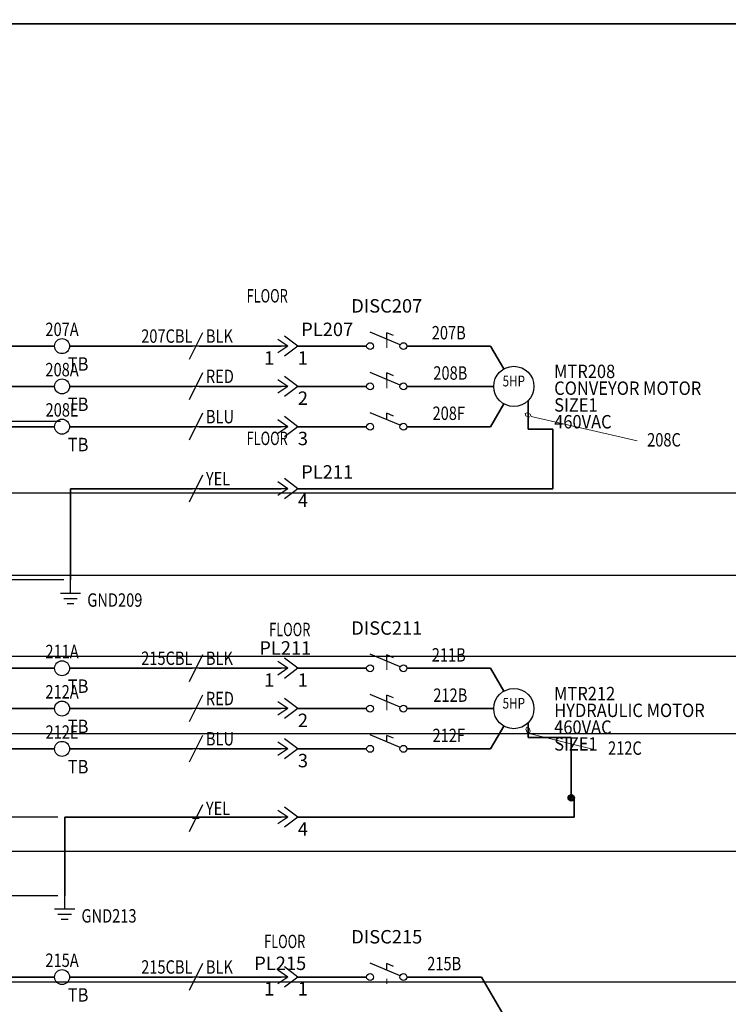
# Model space of a CAD drawing. Extents: x 0 to 33.5, y 0 to 22.4.
# Tile 4 of 8: x 13.3 to 19.9, y 8.5 to 17.7. Entities that reach past the tile are written whole.
import ezdxf
from ezdxf.enums import TextEntityAlignment as Align

# ---------------------------------------------------------------- set-up
doc = ezdxf.new("R2010")
doc.units = 0
doc.header["$MEASUREMENT"] = 0
for name, color, linetype, lineweight in [('A-ANNO-DIMS', 2, 'Continuous', 18), ('LINK', 9, 'Continuous', 18), ('MISC', 7, 'Continuous', 13), ('SYMS', 7, 'Continuous', 25), ('WIRENO', 72, 'Continuous', 18), ('WIRES', 7, 'Continuous', 35)]:
    doc.layers.add(name, color=color, linetype=linetype, lineweight=lineweight)
for name, color, linetype in [('DESC', 150, 'Continuous'), ('DESCCHILD', 20, 'Continuous'), ('TAGS', 150, 'Continuous'), ('TERMS', 123, 'Continuous'), ('WIREREF', 52, 'Continuous')]:
    doc.layers.add(name, color=color, linetype=linetype)
doc.styles.add('WD', font='romans.shx')
doc.dimstyles.get("Standard").update_dxf_attribs({"dimtxt": 0.18, "dimasz": 0.18, "dimexe": 0.18, "dimexo": 0.0625, "dimgap": 0.09, "dimtad": 0, "dimtih": 1, "dimtoh": 1, "dimdec": 4, "dimzin": 0, "dimdsep": 46, "dimtxsty": 'Standard', "dimcen": 0.09, "dimadec": 0, "dimazin": 0, "dimtfac": 1, "dimtdec": 4, "dimtofl": 0, "dimtmove": 0, "dimatfit": 3, "dimfxl": 1, "dimtolj": 1, "dimtzin": 0, "dimarcsym": 0})

# ---------------------------------------------------------------- blocks, each defined once
blk = doc.blocks.new('HT0W02')
blk.add_circle((0, 0), 0.0699)
at = {"style": 'WD'}
for tag, p, width in [('INST', (0.0625, 0.4196), 0.7), ('LOC', (0.0625, 0.25), 0.7), ('DESC1', (0.0532, -0.3851), 0.8)]:
    blk.add_attdef(tag, p, '', height=0.125, dxfattribs=dict(at, width=width))
at = {"style": 'WD', "width": 0.8, "flags": 8}
blk.add_attdef('WIRENO', text='', height=0.125, dxfattribs=at).set_placement((0, 0.0938), align=Align.CENTER)
at = {"style": 'WD', "flags": 1}
for tag, p, height in [('X4TERM01', (-0.0699, 0), 0.0125), ('X4TERMDESC01', (-0.0552, -0.0229), 0.025), ('X2TERMDESC01', (-0.006, 0.0287), 0.025), ('STRIPSEQ', (0, 0), 0.00125), ('X2TERM01', (0, 0.0699), 0.0125), ('X1TERMDESC01', (0.0393, -0.0027), 0.025), ('X1TERM01', (0.0699, 0), 0.0125), ('LINKTERM', (0, -0.0019), 0.00125), ('X8TERM01', (0, -0.0699), 0.0125), ('X8TERMDESC01', (0, -0.0535), 0.025)]:
    blk.add_attdef(tag, p, '', height=height, dxfattribs=at)
at = {"style": 'WD'}
for tag, p, height, width, flags in [('TAGSTRIP', (0.0532, -0.2288), 0.125, 0.9, 8), ('ASSYCODE', (0.0625, -0.2812), 0.01, 0.7, 1), ('CAT', (0.2132, -0.4063), 0.1094, 0.8, 1), ('DESC2', (0.0532, -0.5413), 0.125, 0.8, 8), ('DESC3', (0.0532, -0.6976), 0.125, 0.8, 8)]:
    blk.add_attdef(tag, p, '', height=height, dxfattribs=dict(at, width=width, flags=flags))
at = {"style": 'WD', "width": 0.8, "flags": 1}
blk.add_attdef('MFG', text='', height=0.1094, dxfattribs=at).set_placement((0.0882, -0.4063), align=Align.RIGHT)
blk = doc.blocks.new('HMO13')
blk.add_circle((0, 0), 0.1875)
at = {"style": 'WD'}
for tag, p, width in [('INST', (0.3805, 0.4032), 0.7), ('LOC', (0.3805, 0.2336), 0.7), ('TAG1', (0.375, 0.0774), 0.9), ('DESC1', (0.376, -0.0789), 0.9), ('DESC2', (0.376, -0.2351), 0.9), ('DESC3', (0.376, -0.3914), 0.9), ('RATING3', (0.375, -0.5476), 0.8), ('RATING4', (0.375, -0.7039), 0.8), ('WDTAGALT', (0.375, -0.875), 0.7)]:
    blk.add_attdef(tag, p, '', height=0.125, dxfattribs=dict(at, width=width))
at = {"style": 'WD', "width": 0.8}
blk.add_attdef('RATING1', text='', height=0.1, dxfattribs=at).set_placement((0, 0), align=Align.CENTER)
at = {"style": 'WD', "flags": 1}
for tag, p in [('X0TERM01', (-0.0938, 0.1624)), ('X4TERM02', (-0.1875, 0)), ('X0TERM03', (-0.0938, -0.1624)), ('X0TERM04', (0.1326, -0.1326))]:
    blk.add_attdef(tag, p, '', height=0.0125, dxfattribs=at)
at = {"style": 'WD', "flags": 9}
for tag, p in [('ASSYCODE', (0, 0.125)), ('FAMILY', (-0.0053, 0.1698))]:
    blk.add_attdef(tag, text='', height=0.01, dxfattribs=at).set_placement(p, align=Align.CENTER)
at = {"style": 'WD', "flags": 1}
for tag, p in [('MFG', (0, 0.1404)), ('CAT', (0, 0.1593))]:
    blk.add_attdef(tag, text='', height=0.01, dxfattribs=at).set_placement(p, align=Align.MIDDLE)
at = {"style": 'WD', "width": 0.8}
blk.add_attdef('RATING2', text='', height=0.1, dxfattribs=at).set_placement((0, -0.0312), align=Align.TOP_CENTER)
blk = doc.blocks.new('HDS11')
for p, q in [((0.1257, 0.0127), (-0.1559, 0.1301)), ((0, 0.0651), (0, 0.125)), ((0.0625, 0.099), (0, 0.125))]:
    blk.add_line(p, q)
for centre in [(-0.1553, 0), (0.1553, 0)]:
    blk.add_circle(centre, 0.0322)
at = {"style": 'WD', "width": 0.7}
for tag, p in [('INST', (0, 0.625)), ('LOC', (0, 0.4688)), ('RATING1', (0, 0.1562)), ('XREF', (0, -0.2363)), ('DESC1', (0, -0.4062)), ('DESC2', (0, -0.5625))]:
    blk.add_attdef(tag, text='', height=0.125, dxfattribs=at).set_placement(p, align=Align.CENTER)
at = {"style": 'WD'}
blk.add_attdef('TAG1', text='', height=0.125, dxfattribs=at).set_placement((0, 0.3125), align=Align.CENTER)
for tag, p in [('X2LINK', (0, 0.4375)), ('X8LINK', (0, -0.0156))]:
    blk.add_attdef(tag, p, '', height=0.01, dxfattribs=at)
for tag, p, height, flags in [('FAMILY', (0.2062, 0.1306), 0.01, 9), ('X4TERM01', (-0.1875, 0), 0.0125, 1), ('X1TERM02', (0.1875, 0), 0.0125, 1), ('CONTACT', (0.2062, 0.0401), 0.01, 9)]:
    blk.add_attdef(tag, p, '', height=height, dxfattribs=dict(at, flags=flags))
at = {"style": 'WD', "flags": 9}
for tag, p in [('MFG', (0.2278, 0.0887)), ('CAT', (0.2297, 0.1082)), ('ASSYCODE', (0.2188, 0.0625))]:
    blk.add_attdef(tag, text='', height=0.01, dxfattribs=at).set_placement(p, align=Align.CENTER)
at = {"style": 'WD', "flags": 8}
blk.add_attdef('TERM01', text='', height=0.125, dxfattribs=at).set_placement((-0.25, -0.0314), align=Align.TOP_RIGHT)
blk.add_attdef('TERM02', text='', height=0.125, dxfattribs=at).set_placement((0.25, -0.0314), align=Align.TOP_LEFT)
blk = doc.blocks.new('WDDOT')
for radius in [0.03, 0.0187, 0.00929]:
    blk.add_circle((0, 0), radius)
blk = doc.blocks.new('VGND2')
for p, q in [((0, -0.125), (0, 0)), ((0.09375, -0.125), (-0.09375, -0.125)), ((-0.0625, -0.171875), (0.0625, -0.171875)), ((-0.03125, -0.21875), (0.03125, -0.21875))]:
    blk.add_line(p, q)
at = {"style": 'WD', "width": 0.8}
for tag, p in [('INST', (0.15625, 0.125)), ('LOC', (0.15625, -0.03125)), ('TAG1', (0.15625, -0.1875)), ('DESC1', (0.15625, -0.34375)), ('DESC2', (0.15625, -0.5))]:
    blk.add_attdef(tag, text='', height=0.125, dxfattribs=at).set_placement(p, align=Align.MIDDLE_LEFT)
at = {"style": 'WD', "flags": 1}
for tag in ['ASSYCODE', 'X2TERM01', 'CAT', 'MFG', 'FAMILY']:
    blk.add_attdef(tag, (0, 0), '', height=0.01, dxfattribs=at)
blk = doc.blocks.new('HCN1PJ')
for p, q in [((0.0625, 0), (-0.0625, 0.0938)), ((-0.0312, 0), (-0.125, 0.0625)), ((-0.0312, 0), (-0.125, -0.0625)), ((-0.0312, 0), (-0.0938, 0)), ((0.0625, 0), (-0.0625, -0.0938))]:
    blk.add_line(p, q)
at = {"style": 'WD', "width": 0.7}
for tag, p in [('DESC1', (-0.0312, 0.4062)), ('DESC2', (-0.0312, 0.25))]:
    blk.add_attdef(tag, text='', height=0.125, dxfattribs=at).set_placement(p, align=Align.RIGHT)
for tag, p in [('INST', (0.0938, 0.4062)), ('LOC', (0.0938, 0.25))]:
    blk.add_attdef(tag, p, '', height=0.125, dxfattribs=at)
at = {"style": 'WD'}
for tag, p, height in [('TAG1', (0.0938, 0.0938), 0.125), ('X2LINK', (-0.0625, 0.125), 0.01), ('X8LINK', (-0.0625, -0.125), 0.01)]:
    blk.add_attdef(tag, p, '', height=height, dxfattribs=at)
for tag, p, height, flags in [('WDBLKNAM', (0.0484, 0.1036), 0.01, 9), ('FAMILY', (0.0484, 0.1211), 0.01, 9), ('X4TERMDESC01', (-0.1061, 0.0218), 0.01, 1), ('X4TERM01', (-0.0938, 0), 0.0125, 1), ('X1TERM02', (0.0625, 0), 0.0125, 1), ('X1TERMDESC02', (0.0672, 0.0164), 0.01, 1)]:
    blk.add_attdef(tag, p, '', height=height, dxfattribs=dict(at, flags=flags))
at = {"style": 'WD', "flags": 9}
for tag, p in [('ASSYCODE', (0.0668, 0.0437)), ('MFG', (0.0715, 0.0575)), ('CAT', (0.0735, 0.0769))]:
    blk.add_attdef(tag, text='', height=0.01, dxfattribs=at).set_placement(p, align=Align.CENTER)
at = {"style": 'WD', "flags": 8}
blk.add_attdef('TERM01', text='', height=0.125, dxfattribs=at).set_placement((-0.1562, -0.047), align=Align.TOP_RIGHT)
blk.add_attdef('TERM02', text='', height=0.125, dxfattribs=at).set_placement((0.0625, -0.047), align=Align.TOP_LEFT)
blk = doc.blocks.new('HCN2PJ')
for p, q in [((0.0625, 0), (-0.0625, 0.0938)), ((-0.0312, 0), (-0.125, 0.0625)), ((-0.0312, 0), (-0.125, -0.0625)), ((-0.0312, 0), (-0.0938, 0)), ((0.0625, 0), (-0.0625, -0.0938))]:
    blk.add_line(p, q)
at = {"style": 'WD', "width": 0.7}
for tag, p in [('DESC1', (-0.0312, 0.4062)), ('DESC2', (-0.0312, 0.25))]:
    blk.add_attdef(tag, text='', height=0.125, dxfattribs=at).set_placement(p, align=Align.RIGHT)
for tag, p in [('INST', (0.0938, 0.4062)), ('LOC', (0.0938, 0.25))]:
    blk.add_attdef(tag, p, '', height=0.125, dxfattribs=at)
at = {"style": 'WD'}
for tag, p, height in [('TAG2', (0.0938, 0.0938), 0.125), ('X2LINK', (-0.0625, 0.125), 0.01), ('X8LINK', (-0.0625, -0.125), 0.01)]:
    blk.add_attdef(tag, p, '', height=height, dxfattribs=at)
for tag, p, height, flags in [('FAMILY', (0.0484, 0.1211), 0.01, 9), ('X4TERMDESC01', (-0.1126, 0.0188), 0.01, 1), ('X4TERM01', (-0.0938, 0), 0.0125, 1), ('X1TERM02', (0.0625, 0), 0.0125, 1), ('X1TERMDESC02', (0.0672, 0.0141), 0.01, 1)]:
    blk.add_attdef(tag, p, '', height=height, dxfattribs=dict(at, flags=flags))
at = {"style": 'WD', "flags": 8}
blk.add_attdef('TERM01', text='', height=0.125, dxfattribs=at).set_placement((-0.1562, -0.047), align=Align.TOP_RIGHT)
blk.add_attdef('TERM02', text='', height=0.125, dxfattribs=at).set_placement((0.0625, -0.047), align=Align.TOP_LEFT)
blk = doc.blocks.new('HW01')
for p, q in [((0.0625, 0.125), (-0.0625, -0.125)), ((0.0312, 0), (-0.0312, 0))]:
    blk.add_line(p, q)
at = {"style": 'WD', "width": 0.7, "flags": 1}
for tag, p in [('INST', (0, 0.3571)), ('LOC', (0, 0.1875)), ('XREF', (0, -0.3)), ('DESC1', (0, -0.4563)), ('DESC2', (0, -0.6125))]:
    blk.add_attdef(tag, text='', height=0.125, dxfattribs=at).set_placement(p, align=Align.CENTER)
at = {"style": 'WD', "width": 0.8}
blk.add_attdef('TAG1', text='', height=0.125, dxfattribs=at).set_placement((-0.0312, 0.0312), align=Align.RIGHT)
at = {"style": 'WD'}
for tag, p in [('X2LINK', (0, 0.125)), ('X8LINK', (0, -0.125))]:
    blk.add_attdef(tag, p, '', height=0.01, dxfattribs=at)
at = {"style": 'WD', "flags": 9}
for tag, p in [('FAMILY', (0.0234, 0.1181)), ('ASSYCODE', (0.0286, 0.042))]:
    blk.add_attdef(tag, text='', height=0.01, dxfattribs=at).set_placement(p, align=Align.CENTER)
at = {"style": 'WD', "width": 0.8}
blk.add_attdef('RATING1', (0.0938, 0.0312), '', height=0.125, dxfattribs=at)
at = {"style": 'WD', "flags": 1}
for tag, p in [('X4TERM01', (-0.0312, 0)), ('X1TERM01', (0.0312, 0))]:
    blk.add_attdef(tag, p, '', height=0.0125, dxfattribs=at)
at = {"style": 'WD', "width": 0.8, "flags": 1}
blk.add_attdef('MFG', text='', height=0.0938, dxfattribs=at).set_placement((-0.125, -0.0312), align=Align.TOP_RIGHT)
blk.add_attdef('CAT', text='', height=0.0938, dxfattribs=at).set_placement((0.0312, -0.0312), align=Align.TOP_LEFT)
blk = doc.blocks.new('HW02')
for p, q in [((0.0625, 0.125), (-0.0625, -0.125)), ((0.0312, 0), (-0.0312, 0))]:
    blk.add_line(p, q)
at = {"style": 'WD', "width": 0.7, "flags": 1}
for tag, p in [('INST', (0, 0.3571)), ('LOC', (0, 0.1875)), ('XREF', (0, -0.3)), ('DESC1', (0, -0.4563)), ('DESC2', (0, -0.6125))]:
    blk.add_attdef(tag, text='', height=0.125, dxfattribs=at).set_placement(p, align=Align.CENTER)
at = {"style": 'WD', "width": 0.8}
blk.add_attdef('TAG2', text='', height=0.125, dxfattribs=at).set_placement((-0.0312, 0.0312), align=Align.RIGHT)
at = {"style": 'WD'}
for tag, p in [('X2LINK', (0, 0.125)), ('X8LINK', (0, -0.125))]:
    blk.add_attdef(tag, p, '', height=0.01, dxfattribs=at)
at = {"style": 'WD', "flags": 9}
blk.add_attdef('FAMILY', text='', height=0.01, dxfattribs=at).set_placement((0.0234, 0.1181), align=Align.CENTER)
at = {"style": 'WD', "width": 0.8}
blk.add_attdef('RATING1', (0.0938, 0.0312), '', height=0.125, dxfattribs=at)
at = {"style": 'WD', "flags": 1}
for tag, p in [('X4TERM01', (-0.0312, 0)), ('X1TERM01', (0.0312, 0))]:
    blk.add_attdef(tag, p, '', height=0.0125, dxfattribs=at)
blk = doc.blocks.new('WD_WNV')
at = {"style": 'WD', "flags": 1}
for tag, p in [('W01USER', (-0.0625, 0.0938)), ('W02USER', (-0.0625, 0.0859)), ('W03USER', (-0.0625, 0.0781)), ('W04USER', (-0.0625, 0.0703)), ('W05USER', (-0.0625, 0.0625)), ('W06USER', (-0.0625, 0.0547)), ('W07USER', (-0.0625, 0.0469)), ('W08USER', (-0.0625, 0.0391)), ('W09USER', (-0.0625, 0.0312)), ('W10USER', (-0.0625, 0.0234))]:
    blk.add_attdef(tag, text='', height=0.005, dxfattribs=at).set_placement(p, align=Align.CENTER)
at = {"style": 'WD', "width": 0.8}
blk.add_attdef('WIRENO', text='', height=0.125, dxfattribs=at).set_placement((-0.05, 0), align=Align.MIDDLE_RIGHT)
blk = doc.blocks.new('WD_WNH')
at = {"style": 'WD', "width": 0.8}
blk.add_attdef('WIRENO', text='', height=0.125, dxfattribs=at).set_placement((0, 0.0625), align=Align.CENTER)
at = {"style": 'WD', "flags": 1}
for tag, p in [('W01USER', (0, 0.0781)), ('W02USER', (0, 0.0703)), ('W03USER', (0, 0.0625)), ('W04USER', (0, 0.0547)), ('W05USER', (0, 0.0469)), ('W06USER', (0, 0.0391)), ('W07USER', (0, 0.0312)), ('W08USER', (0, 0.0234)), ('W09USER', (0, 0.0156)), ('W10USER', (0, 0.0078))]:
    blk.add_attdef(tag, text='', height=0.005, dxfattribs=at).set_placement(p, align=Align.CENTER)
blk = doc.blocks.new('*D46')
at = {"layer": 'A-ANNO-DIMS', "color": 0, "lineweight": -2, "transparency": 16777216}
for p, q in [((13.6523, 13.9244), (1.48, 13.9244)), ((1.66, 13.7444), (1.66, 13.3662)), ((1.66, 12.628), (1.66, 13.0062)), ((13.6816, 12.448), (1.48, 12.448))]:
    blk.add_line(p, q, dxfattribs=at)
at = {"layer": 'A-ANNO-DIMS', "color": 0, "transparency": 16777216}
for points in [[(1.63, 13.7444), (1.69, 13.7444), (1.66, 13.9244)], [(1.63, 12.628), (1.69, 12.628), (1.66, 12.448)]]:
    blk.add_solid(points, dxfattribs=at)
at = {"layer": 'Defpoints', "color": 0, "transparency": 16777216}
for p in [(13.7148, 13.9244), (1.66, 12.448), (13.7441, 12.448)]:
    blk.add_point(p, dxfattribs=at)
at = {"layer": 'A-ANNO-DIMS', "color": 0, "transparency": 16777216, "insert": (1.66, 13.1862), "char_height": 0.18, "attachment_point": 5}
blk.add_mtext('\\A1;1.48', dxfattribs=at)
blk = doc.blocks.new('*D47')
at = {"layer": 'A-ANNO-DIMS', "color": 0, "lineweight": -2, "transparency": 16777216}
for p, q in [((13.627211, 10.238995), (1.48, 10.238995)), ((1.66, 10.058995), (1.66, 9.686874)), ((13.627211, 9.506874), (1.48, 9.506874)), ((1.66, 9.506874), (1.66, 9.326874)), ((1.66, 9.326874), (1.48, 9.326874))]:
    blk.add_line(p, q, dxfattribs=at)
at = {"layer": 'A-ANNO-DIMS', "color": 0, "transparency": 16777216}
for points in [[(1.63, 10.058995), (1.69, 10.058995), (1.66, 10.238995)], [(1.63, 9.686874), (1.69, 9.686874), (1.66, 9.506874)]]:
    blk.add_solid(points, dxfattribs=at)
at = {"layer": 'Defpoints', "color": 0, "transparency": 16777216}
for p in [(13.689711, 10.238995), (1.66, 9.506874), (13.689711, 9.506874)]:
    blk.add_point(p, dxfattribs=at)
at = {"layer": 'A-ANNO-DIMS', "color": 0, "transparency": 16777216, "insert": (1.135, 9.326874), "char_height": 0.18, "attachment_point": 5}
blk.add_mtext('\\A1;0.73', dxfattribs=at)
blk = doc.blocks.new('*D56')
at = {"layer": 'A-ANNO-DIMS', "color": 0, "lineweight": -2, "transparency": 16777216}
for p, q in [((29.389766, 13.255775), (1.48, 13.255775)), ((1.66, 13.075775), (1.66, 12.669774)), ((29.4322, 12.489774), (1.48, 12.489774)), ((1.66, 12.489774), (1.66, 12.309774)), ((1.66, 12.309774), (1.48, 12.309774))]:
    blk.add_line(p, q, dxfattribs=at)
at = {"layer": 'A-ANNO-DIMS', "color": 0, "transparency": 16777216}
for points in [[(1.63, 13.075775), (1.69, 13.075775), (1.66, 13.255775)], [(1.63, 12.669774), (1.69, 12.669774), (1.66, 12.489774)]]:
    blk.add_solid(points, dxfattribs=at)
at = {"layer": 'Defpoints', "color": 0, "transparency": 16777216}
for p in [(29.452266, 13.255775), (1.66, 12.489774), (29.4947, 12.489774)]:
    blk.add_point(p, dxfattribs=at)
at = {"layer": 'A-ANNO-DIMS', "color": 0, "transparency": 16777216, "insert": (1.045, 12.309774), "char_height": 0.18, "attachment_point": 5}
blk.add_mtext('\\A1;0.766', dxfattribs=at)
blk = doc.blocks.new('*D57')
at = {"layer": 'A-ANNO-DIMS', "color": 0, "lineweight": -2, "transparency": 16777216}
for p, q in [((29.4322, 12.489774), (1.48, 12.489774)), ((1.66, 12.309774), (1.66, 11.913516)), ((29.435818, 11.733516), (1.48, 11.733516)), ((1.66, 11.733516), (1.66, 11.553516)), ((1.66, 11.553516), (1.48, 11.553516))]:
    blk.add_line(p, q, dxfattribs=at)
at = {"layer": 'A-ANNO-DIMS', "color": 0, "transparency": 16777216}
for points in [[(1.63, 12.309774), (1.69, 12.309774), (1.66, 12.489774)], [(1.63, 11.913516), (1.69, 11.913516), (1.66, 11.733516)]]:
    blk.add_solid(points, dxfattribs=at)
at = {"layer": 'Defpoints', "color": 0, "transparency": 16777216}
for p in [(29.4947, 12.489774), (1.66, 11.733516), (29.498318, 11.733516)]:
    blk.add_point(p, dxfattribs=at)
at = {"layer": 'A-ANNO-DIMS', "color": 0, "transparency": 16777216, "insert": (1.135, 11.553516), "char_height": 0.18, "attachment_point": 5}
blk.add_mtext('\\A1;0.76', dxfattribs=at)
blk = doc.blocks.new('*D58')
at = {"layer": 'A-ANNO-DIMS', "color": 0, "lineweight": -2, "transparency": 16777216}
for p, q in [((29.435818, 11.733516), (1.48, 11.733516)), ((1.66, 11.553516), (1.66, 11.194575)), ((29.438773, 11.014575), (1.48, 11.014575)), ((1.66, 11.014575), (1.66, 10.834575)), ((1.66, 10.834575), (1.48, 10.834575))]:
    blk.add_line(p, q, dxfattribs=at)
at = {"layer": 'A-ANNO-DIMS', "color": 0, "transparency": 16777216}
for points in [[(1.63, 11.553516), (1.69, 11.553516), (1.66, 11.733516)], [(1.63, 11.194575), (1.69, 11.194575), (1.66, 11.014575)]]:
    blk.add_solid(points, dxfattribs=at)
at = {"layer": 'Defpoints', "color": 0, "transparency": 16777216}
for p in [(29.498318, 11.733516), (1.66, 11.014575), (29.501273, 11.014575)]:
    blk.add_point(p, dxfattribs=at)
at = {"layer": 'A-ANNO-DIMS', "color": 0, "transparency": 16777216, "insert": (1.075, 10.834575), "char_height": 0.18, "attachment_point": 5}
blk.add_mtext('\\A1;0.719', dxfattribs=at)
blk = doc.blocks.new('*D59')
at = {"layer": 'A-ANNO-DIMS', "color": 0, "lineweight": -2, "transparency": 16777216}
for p, q in [((29.438773, 11.014575), (1.48, 11.014575)), ((1.66, 10.834575), (1.66, 10.646575)), ((1.66, 10.098575), (1.66, 10.286575)), ((29.435818, 9.918575), (1.48, 9.918575))]:
    blk.add_line(p, q, dxfattribs=at)
at = {"layer": 'A-ANNO-DIMS', "color": 0, "transparency": 16777216}
for points in [[(1.63, 10.834575), (1.69, 10.834575), (1.66, 11.014575)], [(1.63, 10.098575), (1.69, 10.098575), (1.66, 9.918575)]]:
    blk.add_solid(points, dxfattribs=at)
at = {"layer": 'Defpoints', "color": 0, "transparency": 16777216}
for p in [(29.501273, 11.014575), (1.66, 9.918575), (29.498318, 9.918575)]:
    blk.add_point(p, dxfattribs=at)
at = {"layer": 'A-ANNO-DIMS', "color": 0, "transparency": 16777216, "insert": (1.66, 10.466575), "char_height": 0.18, "attachment_point": 5}
blk.add_mtext('\\A1;1.096', dxfattribs=at)
blk = doc.blocks.new('*D60')
at = {"layer": 'A-ANNO-DIMS', "color": 0, "lineweight": -2, "transparency": 16777216}
for p, q in [((29.435818, 9.918575), (1.48, 9.918575)), ((1.66, 9.738575), (1.66, 9.490438)), ((1.66, 8.882301), (1.66, 9.130438)), ((29.4322, 8.702301), (1.48, 8.702301))]:
    blk.add_line(p, q, dxfattribs=at)
at = {"layer": 'A-ANNO-DIMS', "color": 0, "transparency": 16777216}
for points in [[(1.63, 9.738575), (1.69, 9.738575), (1.66, 9.918575)], [(1.63, 8.882301), (1.69, 8.882301), (1.66, 8.702301)]]:
    blk.add_solid(points, dxfattribs=at)
at = {"layer": 'Defpoints', "color": 0, "transparency": 16777216}
for p in [(29.498318, 9.918575), (1.66, 8.702301), (29.4947, 8.702301)]:
    blk.add_point(p, dxfattribs=at)
at = {"layer": 'A-ANNO-DIMS', "color": 0, "transparency": 16777216, "insert": (1.66, 9.310438), "char_height": 0.18, "attachment_point": 5}
blk.add_mtext('\\A1;1.22', dxfattribs=at)
blk = doc.blocks.new('*D61')
at = {"layer": 'A-ANNO-DIMS', "color": 0, "lineweight": -2, "transparency": 16777216}
for p, q in [((23.0885, 18.3786), (1.48, 18.3786)), ((1.66, 18.1986), (1.66, 15.9972)), ((1.66, 13.4358), (1.66, 15.6372)), ((20.8383, 13.2558), (1.48, 13.2558))]:
    blk.add_line(p, q, dxfattribs=at)
at = {"layer": 'A-ANNO-DIMS', "color": 0, "transparency": 16777216}
for points in [[(1.63, 18.1986), (1.69, 18.1986), (1.66, 18.3786)], [(1.63, 13.4358), (1.69, 13.4358), (1.66, 13.2558)]]:
    blk.add_solid(points, dxfattribs=at)
at = {"layer": 'Defpoints', "color": 0, "transparency": 16777216}
for p in [(23.151, 18.3786), (1.66, 13.2558), (20.9008, 13.2558)]:
    blk.add_point(p, dxfattribs=at)
at = {"layer": 'A-ANNO-DIMS', "color": 0, "transparency": 16777216, "insert": (1.66, 15.8172), "char_height": 0.18, "attachment_point": 5}
blk.add_mtext('\\A1;5.123', dxfattribs=at)

msp = doc.modelspace()

# ---------------------------------------------------------------- linework, layer by layer
at = {"layer": 'LINK'}
for points in [[(16.6912, 14.6094), (16.6912, 14.6875)], [(16.6912, 14.2344), (16.6912, 14.3125)], [(16.6912, 11.6094), (16.6912, 11.6875)], [(16.6912, 11.2344), (16.6912, 11.3125)], [(16.6912, 8.7344), (16.6912, 8.6875)]]:
    msp.add_lwpolyline(points, dxfattribs=at)
at = {"layer": 'WIRENO'}
for points in [[(19.0239, 13.7421), (18.0359, 13.9707), (18.0284, 13.9914), (18.0001, 14.0047), (17.9793, 13.9972), (17.9868, 13.9764), (18.0151, 13.9632), (18.0255, 13.9669)], [(18.6455, 10.8623), (18.0178, 11.019), (18.0275, 11.0389), (18.0172, 11.0684), (17.9974, 11.078), (17.9877, 11.0582), (17.9979, 11.0286), (18.0079, 11.0238)]]:
    msp.add_lwpolyline(points, dxfattribs=at)
at = {"layer": 'WIRES'}
for p, q in [((5.1875, 17.625), (30.0939, 17.625)), ((11.3605, 14.625), (13.5956, 14.625)), ((13.7353, 14.625), (14.8807, 14.625)), ((14.9432, 14.625), (15.7062, 14.625)), ((15.8625, 14.625), (16.5036, 14.625)), ((16.8786, 14.625), (17.6585, 14.625)), ((17.6585, 14.625), (17.7812, 14.4124)), ((11.3605, 14.25), (13.5956, 14.25)), ((13.7353, 14.25), (14.8807, 14.25)), ((14.9432, 14.25), (15.7062, 14.25)), ((15.8625, 14.25), (16.5036, 14.25)), ((16.8786, 14.25), (17.6875, 14.25)), ((17.6585, 13.875), (17.7812, 14.0876)), ((18.0076, 13.8505), (18.0076, 14.1174)), ((11.3605, 13.875), (13.5956, 13.875)), ((13.7353, 13.875), (14.8807, 13.875)), ((14.9432, 13.875), (15.7062, 13.875)), ((15.8625, 13.875), (16.5036, 13.875)), ((16.8786, 13.875), (17.6585, 13.875)), ((18.2389, 13.8505), (18.0076, 13.8505)), ((18.2389, 13.2976), (18.2389, 13.8505)), ((13.7441, 12.448), (13.7441, 13.2976)), ((13.7441, 13.2976), (14.8807, 13.2976)), ((14.9432, 13.2976), (15.7062, 13.2976)), ((15.8625, 13.2976), (18.2389, 13.2976)), ((11.3605, 11.625), (13.5956, 11.625)), ((13.7353, 11.625), (14.8807, 11.625)), ((14.9432, 11.625), (15.7062, 11.625)), ((15.8625, 11.625), (16.5036, 11.625)), ((16.8786, 11.625), (17.6585, 11.625)), ((17.6585, 11.625), (17.7812, 11.4124)), ((11.3605, 11.25), (13.5956, 11.25)), ((13.7353, 11.25), (14.8807, 11.25)), ((14.9432, 11.25), (15.7062, 11.25)), ((15.8625, 11.25), (16.5036, 11.25)), ((16.8786, 11.25), (17.6875, 11.25)), ((18.0076, 10.9796), (18.0076, 11.1174)), ((17.6585, 10.875), (17.7812, 11.0876)), ((18.4103, 10.9796), (18.0076, 10.9796)), ((18.4103, 10.4178), (18.4103, 10.9796)), ((11.3605, 10.875), (13.5956, 10.875)), ((13.7353, 10.875), (14.8807, 10.875)), ((14.9432, 10.875), (15.7062, 10.875)), ((15.8625, 10.875), (16.5036, 10.875)), ((16.8786, 10.875), (17.6585, 10.875)), ((18.4359, 10.4178), (18.4103, 10.4178)), ((18.4359, 10.239), (18.4359, 10.4178)), ((13.6897, 9.5069), (13.6897, 10.239)), ((13.6897, 10.239), (15.7062, 10.239)), ((15.8625, 10.239), (18.4359, 10.239)), ((11.3605, 8.75), (13.5956, 8.75)), ((13.7353, 8.75), (14.8807, 8.75)), ((14.9432, 8.75), (15.7062, 8.75)), ((15.8625, 8.75), (16.5036, 8.75)), ((16.8786, 8.75), (17.5742, 8.75)), ((17.5742, 8.75), (17.7691, 8.4124))]:
    msp.add_line(p, q, dxfattribs=at)

# ---------------------------------------------------------------- block references
at = {"layer": 'SYMS'}
ref = msp.add_blockref('HCN1PJ', (15.8, 14.625), dxfattribs=at)
ref.add_attrib('DESC1', 'FLOOR', dxfattribs={"layer": 'DESC', "height": 0.125, "style": 'WD', "width": 0.7}).set_placement((15.7687, 15.0312), align=Align.RIGHT)
ref.add_attrib('TAG1', 'PL207', (15.8937, 14.7188), dxfattribs={"layer": 'TAGS', "height": 0.125, "style": 'WD'})
ref.add_attrib('TERM01', '1', dxfattribs={"layer": 'TERMS', "linetype": 'Continuous', "height": 0.125, "style": 'WD', "flags": 8}).set_placement((15.6437, 14.578), align=Align.TOP_RIGHT)
ref.add_attrib('TERM02', '1', dxfattribs={"layer": 'TERMS', "linetype": 'Continuous', "height": 0.125, "style": 'WD', "flags": 8}).set_placement((15.8625, 14.578), align=Align.TOP_LEFT)
ref = msp.add_blockref('HDS11', (16.6911, 14.625), dxfattribs=at)
ref.add_attrib('TAG1', 'DISC207', dxfattribs={"layer": 'TAGS', "height": 0.125, "style": 'WD'}).set_placement((16.6911, 14.9375), align=Align.CENTER)
ref = msp.add_blockref('HT0W02', (13.6654, 14.625), dxfattribs=at)
ref.add_attrib('WIRENO', '207A', dxfattribs={"layer": 'WIREREF', "linetype": 'Continuous', "height": 0.125, "style": 'WD', "width": 0.8, "flags": 8}).set_placement((13.6654, 14.7188), align=Align.CENTER)
ref.add_attrib('TAGSTRIP', 'TB', (13.7186, 14.3962), dxfattribs={"layer": 'TAGS', "linetype": 'Continuous', "height": 0.125, "style": 'WD', "width": 0.9, "flags": 8})
ref = msp.add_blockref('HW01', (14.912, 14.625), dxfattribs=at)
ref.add_attrib('RATING1', 'BLK', (15.0057, 14.6562), dxfattribs={"layer": 'MISC', "height": 0.125, "style": 'WD', "width": 0.8})
ref.add_attrib('TAG1', '207CBL', dxfattribs={"layer": 'TAGS', "height": 0.125, "style": 'WD', "width": 0.8}).set_placement((14.8807, 14.6562), align=Align.RIGHT)
ref = msp.add_blockref('HT0W02', (13.6654, 14.25), dxfattribs=at)
ref.add_attrib('WIRENO', '208A', dxfattribs={"layer": 'WIREREF', "linetype": 'Continuous', "height": 0.125, "style": 'WD', "width": 0.8, "flags": 8}).set_placement((13.6654, 14.3438), align=Align.CENTER)
ref.add_attrib('TAGSTRIP', 'TB', (13.7186, 14.0212), dxfattribs={"layer": 'TAGS', "linetype": 'Continuous', "height": 0.125, "style": 'WD', "width": 0.9, "flags": 8})
ref = msp.add_blockref('HW02', (14.912, 14.25), dxfattribs=at)
ref.add_attrib('RATING1', 'RED', (15.0057, 14.2812), dxfattribs={"layer": 'MISC', "height": 0.125, "style": 'WD', "width": 0.8})
ref = msp.add_blockref('HMO13', (17.875, 14.25), dxfattribs=at)
ref.add_attrib('DESC3', '460VAC', (18.251, 13.8586), dxfattribs={"layer": 'DESC', "height": 0.125, "style": 'WD', "width": 0.9})
ref.add_attrib('RATING1', '5HP', dxfattribs={"layer": 'MISC', "height": 0.1, "style": 'WD', "width": 0.8}).set_placement((17.875, 14.25), align=Align.CENTER)
ref.add_attrib('DESC1', 'CONVEYOR MOTOR', (18.251, 14.1711), dxfattribs={"layer": 'DESC', "height": 0.125, "style": 'WD', "width": 0.9})
ref.add_attrib('DESC2', 'SIZE1', (18.251, 14.0149), dxfattribs={"layer": 'DESC', "height": 0.125, "style": 'WD', "width": 0.9})
ref.add_attrib('TAG1', 'MTR208', (18.25, 14.3274), dxfattribs={"layer": 'TAGS', "height": 0.125, "style": 'WD', "width": 0.9})
ref = msp.add_blockref('HCN2PJ', (15.8, 14.25), dxfattribs=at)
ref.add_attrib('TERM02', '2', dxfattribs={"layer": 'TERMS', "linetype": 'Continuous', "height": 0.125, "style": 'WD', "flags": 8}).set_placement((15.8625, 14.203), align=Align.TOP_LEFT)
for name, p in [('HDS11', (16.6911, 14.25)), ('HDS11', (16.6911, 13.875)), ('HDS11', (16.6911, 11.25)), ('HDS11', (16.6911, 10.875)), ('WDDOT', (18.4103, 10.4178))]:
    msp.add_blockref(name, p, dxfattribs=at)
ref = msp.add_blockref('HT0W02', (13.6654, 13.875), dxfattribs=at)
ref.add_attrib('WIRENO', '208E', dxfattribs={"layer": 'WIREREF', "linetype": 'Continuous', "height": 0.125, "style": 'WD', "width": 0.8, "flags": 8}).set_placement((13.6654, 13.9688), align=Align.CENTER)
ref.add_attrib('TAGSTRIP', 'TB', (13.7186, 13.6462), dxfattribs={"layer": 'TAGS', "linetype": 'Continuous', "height": 0.125, "style": 'WD', "width": 0.9, "flags": 8})
ref = msp.add_blockref('HW02', (14.912, 13.875), dxfattribs=at)
ref.add_attrib('RATING1', 'BLU', (15.0057, 13.9062), dxfattribs={"layer": 'MISC', "height": 0.125, "style": 'WD', "width": 0.8})
ref = msp.add_blockref('HCN2PJ', (15.8, 13.875), dxfattribs=at)
ref.add_attrib('TERM02', '3', dxfattribs={"layer": 'TERMS', "linetype": 'Continuous', "height": 0.125, "style": 'WD', "flags": 8}).set_placement((15.8625, 13.828), align=Align.TOP_LEFT)
ref = msp.add_blockref('HCN2PJ', (15.8, 13.2976), dxfattribs=at)
ref.add_attrib('DESC1', 'FLOOR', dxfattribs={"layer": 'DESCCHILD', "height": 0.125, "style": 'WD', "width": 0.7}).set_placement((15.7687, 13.7038), align=Align.RIGHT)
ref.add_attrib('TAG2', 'PL211', (15.8937, 13.3913), dxfattribs={"layer": 'TAGS', "height": 0.125, "style": 'WD'})
ref.add_attrib('TERM02', '4', dxfattribs={"layer": 'TERMS', "linetype": 'Continuous', "height": 0.125, "style": 'WD', "flags": 8}).set_placement((15.8625, 13.2506), align=Align.TOP_LEFT)
ref = msp.add_blockref('HW02', (14.912, 13.2976), dxfattribs=at)
ref.add_attrib('RATING1', 'YEL', (15.0057, 13.3288), dxfattribs={"layer": 'MISC', "height": 0.125, "style": 'WD', "width": 0.8})
ref = msp.add_blockref('VGND2', (13.7441, 12.448), dxfattribs=at)
ref.add_attrib('TAG1', 'GND209', dxfattribs={"layer": 'TAGS', "height": 0.125, "style": 'WD', "width": 0.8}).set_placement((13.9004, 12.2605), align=Align.MIDDLE_LEFT)
ref = msp.add_blockref('HCN2PJ', (15.8, 10.875), dxfattribs=at)
ref.add_attrib('DESC1', 'FLOOR', dxfattribs={"layer": 'DESCCHILD', "height": 0.125, "style": 'WD', "width": 0.7}).set_placement((15.9789, 11.9241), align=Align.RIGHT)
ref.add_attrib('TAG2', 'PL211', (15.5035, 11.7522), dxfattribs={"layer": 'TAGS', "height": 0.125, "style": 'WD'})
ref.add_attrib('TERM02', '3', dxfattribs={"layer": 'TERMS', "linetype": 'Continuous', "height": 0.125, "style": 'WD', "flags": 8}).set_placement((15.8625, 10.828), align=Align.TOP_LEFT)
ref = msp.add_blockref('HDS11', (16.6911, 11.625), dxfattribs=at)
ref.add_attrib('TAG1', 'DISC211', dxfattribs={"layer": 'TAGS', "height": 0.125, "style": 'WD'}).set_placement((16.6911, 11.9375), align=Align.CENTER)
ref = msp.add_blockref('HT0W02', (13.6654, 11.625), dxfattribs=at)
ref.add_attrib('WIRENO', '211A', dxfattribs={"layer": 'WIREREF', "linetype": 'Continuous', "height": 0.125, "style": 'WD', "width": 0.8, "flags": 8}).set_placement((13.6654, 11.7188), align=Align.CENTER)
ref.add_attrib('TAGSTRIP', 'TB', (13.7186, 11.3962), dxfattribs={"layer": 'TAGS', "linetype": 'Continuous', "height": 0.125, "style": 'WD', "width": 0.9, "flags": 8})
ref = msp.add_blockref('HW02', (14.912, 11.625), dxfattribs=at)
ref.add_attrib('RATING1', 'BLK', (15.0057, 11.6562), dxfattribs={"layer": 'MISC', "height": 0.125, "style": 'WD', "width": 0.8})
ref.add_attrib('TAG2', '215CBL', dxfattribs={"layer": 'TAGS', "height": 0.125, "style": 'WD', "width": 0.8}).set_placement((14.8807, 11.6562), align=Align.RIGHT)
ref = msp.add_blockref('HCN2PJ', (15.8, 11.625), dxfattribs=at)
ref.add_attrib('TERM01', '1', dxfattribs={"layer": 'TERMS', "linetype": 'Continuous', "height": 0.125, "style": 'WD', "flags": 8}).set_placement((15.6437, 11.578), align=Align.TOP_RIGHT)
ref.add_attrib('TERM02', '1', dxfattribs={"layer": 'TERMS', "linetype": 'Continuous', "height": 0.125, "style": 'WD', "flags": 8}).set_placement((15.8625, 11.578), align=Align.TOP_LEFT)
ref = msp.add_blockref('HT0W02', (13.6654, 11.25), dxfattribs=at)
ref.add_attrib('WIRENO', '212A', dxfattribs={"layer": 'WIREREF', "linetype": 'Continuous', "height": 0.125, "style": 'WD', "width": 0.8, "flags": 8}).set_placement((13.6654, 11.3438), align=Align.CENTER)
ref.add_attrib('TAGSTRIP', 'TB', (13.7186, 11.0212), dxfattribs={"layer": 'TAGS', "linetype": 'Continuous', "height": 0.125, "style": 'WD', "width": 0.9, "flags": 8})
ref = msp.add_blockref('HW02', (14.912, 11.25), dxfattribs=at)
ref.add_attrib('RATING1', 'RED', (15.0057, 11.2812), dxfattribs={"layer": 'MISC', "height": 0.125, "style": 'WD', "width": 0.8})
ref = msp.add_blockref('HMO13', (17.875, 11.25), dxfattribs=at)
ref.add_attrib('DESC3', 'SIZE1', (18.251, 10.8586), dxfattribs={"layer": 'DESC', "height": 0.125, "style": 'WD', "width": 0.9})
ref.add_attrib('RATING1', '5HP', dxfattribs={"layer": 'MISC', "height": 0.1, "style": 'WD', "width": 0.8}).set_placement((17.875, 11.25), align=Align.CENTER)
ref.add_attrib('DESC1', 'HYDRAULIC MOTOR', (18.251, 11.1711), dxfattribs={"layer": 'DESC', "height": 0.125, "style": 'WD', "width": 0.9})
ref.add_attrib('DESC2', '460VAC', (18.251, 11.0149), dxfattribs={"layer": 'DESC', "height": 0.125, "style": 'WD', "width": 0.9})
ref.add_attrib('TAG1', 'MTR212', (18.25, 11.3274), dxfattribs={"layer": 'TAGS', "height": 0.125, "style": 'WD', "width": 0.9})
ref = msp.add_blockref('HCN2PJ', (15.8, 11.25), dxfattribs=at)
ref.add_attrib('TERM02', '2', dxfattribs={"layer": 'TERMS', "linetype": 'Continuous', "height": 0.125, "style": 'WD', "flags": 8}).set_placement((15.8625, 11.203), align=Align.TOP_LEFT)
ref = msp.add_blockref('HT0W02', (13.6654, 10.875), dxfattribs=at)
ref.add_attrib('WIRENO', '212E', dxfattribs={"layer": 'WIREREF', "linetype": 'Continuous', "height": 0.125, "style": 'WD', "width": 0.8, "flags": 8}).set_placement((13.6654, 10.9688), align=Align.CENTER)
ref.add_attrib('TAGSTRIP', 'TB', (13.7186, 10.6462), dxfattribs={"layer": 'TAGS', "linetype": 'Continuous', "height": 0.125, "style": 'WD', "width": 0.9, "flags": 8})
ref = msp.add_blockref('HW02', (14.912, 10.875), dxfattribs=at)
ref.add_attrib('RATING1', 'BLU', (15.0057, 10.9062), dxfattribs={"layer": 'MISC', "height": 0.125, "style": 'WD', "width": 0.8})
ref = msp.add_blockref('HW02', (14.912, 10.2275), dxfattribs=at)
ref.add_attrib('RATING1', 'YEL', (15.0057, 10.2587), dxfattribs={"layer": 'MISC', "height": 0.125, "style": 'WD', "width": 0.8})
ref = msp.add_blockref('HCN2PJ', (15.8, 10.239), dxfattribs=at)
ref.add_attrib('TERM02', '4', dxfattribs={"layer": 'TERMS', "linetype": 'Continuous', "height": 0.125, "style": 'WD', "flags": 8}).set_placement((15.8625, 10.192), align=Align.TOP_LEFT)
ref = msp.add_blockref('VGND2', (13.6897, 9.5069), dxfattribs=at)
ref.add_attrib('TAG1', 'GND213', dxfattribs={"layer": 'TAGS', "height": 0.125, "style": 'WD', "width": 0.8}).set_placement((13.846, 9.3194), align=Align.MIDDLE_LEFT)
ref = msp.add_blockref('HDS11', (16.6911, 8.75), dxfattribs=at)
ref.add_attrib('TAG1', 'DISC215', dxfattribs={"layer": 'TAGS', "height": 0.125, "style": 'WD'}).set_placement((16.6911, 9.0625), align=Align.CENTER)
ref = msp.add_blockref('HCN2PJ', (15.8, 8.75), dxfattribs=at)
ref.add_attrib('DESC1', 'FLOOR', dxfattribs={"layer": 'DESCCHILD', "height": 0.125, "style": 'WD', "width": 0.7}).set_placement((15.932, 9.019), align=Align.RIGHT)
ref.add_attrib('TAG2', 'PL215', (15.4559, 8.8155), dxfattribs={"layer": 'TAGS', "height": 0.125, "style": 'WD'})
ref.add_attrib('TERM01', '1', dxfattribs={"layer": 'TERMS', "linetype": 'Continuous', "height": 0.125, "style": 'WD', "flags": 8}).set_placement((15.6437, 8.703), align=Align.TOP_RIGHT)
ref.add_attrib('TERM02', '1', dxfattribs={"layer": 'TERMS', "linetype": 'Continuous', "height": 0.125, "style": 'WD', "flags": 8}).set_placement((15.8625, 8.703), align=Align.TOP_LEFT)
ref = msp.add_blockref('HT0W02', (13.6654, 8.75), dxfattribs=at)
ref.add_attrib('WIRENO', '215A', dxfattribs={"layer": 'WIREREF', "linetype": 'Continuous', "height": 0.125, "style": 'WD', "width": 0.8, "flags": 8}).set_placement((13.6654, 8.8438), align=Align.CENTER)
ref.add_attrib('TAGSTRIP', 'TB', (13.7186, 8.5212), dxfattribs={"layer": 'TAGS', "linetype": 'Continuous', "height": 0.125, "style": 'WD', "width": 0.9, "flags": 8})
ref = msp.add_blockref('HW02', (14.912, 8.75), dxfattribs=at)
ref.add_attrib('RATING1', 'BLK', (15.0057, 8.7812), dxfattribs={"layer": 'MISC', "height": 0.125, "style": 'WD', "width": 0.8})
ref.add_attrib('TAG2', '215CBL', dxfattribs={"layer": 'TAGS', "height": 0.125, "style": 'WD', "width": 0.8}).set_placement((14.8807, 8.7812), align=Align.RIGHT)
at = {"layer": 'WIRENO'}
ref = msp.add_blockref('WD_WNH', (17.2686, 14.625), dxfattribs=at)
ref.add_attrib('WIRENO', '207B', dxfattribs={"linetype": 'Continuous', "height": 0.125, "style": 'WD', "width": 0.8}).set_placement((17.2686, 14.6875), align=Align.CENTER)
ref = msp.add_blockref('WD_WNH', (17.2831, 14.25), dxfattribs=at)
ref.add_attrib('WIRENO', '208B', dxfattribs={"linetype": 'Continuous', "height": 0.125, "style": 'WD', "width": 0.8}).set_placement((17.2831, 14.3125), align=Align.CENTER)
ref = msp.add_blockref('WD_WNH', (17.2686, 13.875), dxfattribs=at)
ref.add_attrib('WIRENO', '208F', dxfattribs={"linetype": 'Continuous', "height": 0.125, "style": 'WD', "width": 0.8}).set_placement((17.2686, 13.9375), align=Align.CENTER)
ref = msp.add_blockref('WD_WNV', (18.0076, 13.9839), dxfattribs=at)
ref.add_attrib('WIRENO', '208C', dxfattribs={"linetype": 'Continuous', "height": 0.125, "style": 'WD', "width": 0.8}).set_placement((19.1172, 13.7528), align=Align.MIDDLE_LEFT)
ref = msp.add_blockref('WD_WNH', (17.2686, 11.625), dxfattribs=at)
ref.add_attrib('WIRENO', '211B', dxfattribs={"linetype": 'Continuous', "height": 0.125, "style": 'WD', "width": 0.8}).set_placement((17.2686, 11.6875), align=Align.CENTER)
ref = msp.add_blockref('WD_WNH', (17.2831, 11.25), dxfattribs=at)
ref.add_attrib('WIRENO', '212B', dxfattribs={"linetype": 'Continuous', "height": 0.125, "style": 'WD', "width": 0.8}).set_placement((17.2831, 11.3125), align=Align.CENTER)
ref = msp.add_blockref('WD_WNH', (17.2686, 10.875), dxfattribs=at)
ref.add_attrib('WIRENO', '212F', dxfattribs={"linetype": 'Continuous', "height": 0.125, "style": 'WD', "width": 0.8}).set_placement((17.2686, 10.9375), align=Align.CENTER)
ref = msp.add_blockref('WD_WNV', (18.0076, 11.0485), dxfattribs=at)
ref.add_attrib('WIRENO', '212C', dxfattribs={"linetype": 'Continuous', "height": 0.125, "style": 'WD', "width": 0.8}).set_placement((18.753, 10.882), align=Align.MIDDLE_LEFT)
ref = msp.add_blockref('WD_WNH', (17.2264, 8.75), dxfattribs=at)
ref.add_attrib('WIRENO', '215B', dxfattribs={"linetype": 'Continuous', "height": 0.125, "style": 'WD', "width": 0.8}).set_placement((17.2264, 8.8125), align=Align.CENTER)

# ---------------------------------------------------------------- dimensions: what is measured, and where the dimension line sits
at = {"layer": 'A-ANNO-DIMS'}
for base, p1, p2, override, picture, middle in [((1.66, 13.2558), (23.151, 18.3786), (20.9008, 13.2558), {"dimdec": 3, "dimlfac": 1, "dimrnd": 0, "dimzin": 0, "dimdsep": 46, "dimlunit": 2}, '*D61', (1.66, 15.8172)), ((1.66, 12.448), (13.7148, 13.9244), (13.7441, 12.448), {"dimdec": 2, "dimlfac": 1, "dimrnd": 0, "dimzin": 0, "dimdsep": 46, "dimlunit": 2}, '*D46', (1.66, 13.1862)), ((1.66, 12.4898), (29.4523, 13.2558), (29.4947, 12.4898), {"dimdec": 3, "dimlfac": 1, "dimrnd": 0, "dimzin": 0, "dimdsep": 46, "dimlunit": 2}, '*D56', (1.045, 12.3098)), ((1.66, 11.7335), (29.4947, 12.4898), (29.4983, 11.7335), {"dimdec": 2, "dimlfac": 1, "dimrnd": 0, "dimzin": 0, "dimdsep": 46, "dimlunit": 2}, '*D57', (1.135, 11.5535)), ((1.66, 11.0146), (29.4983, 11.7335), (29.5013, 11.0146), {"dimdec": 3, "dimlfac": 1, "dimrnd": 0, "dimzin": 0, "dimdsep": 46, "dimlunit": 2}, '*D58', (1.075, 10.8346)), ((1.66, 9.9186), (29.5013, 11.0146), (29.4983, 9.9186), {"dimdec": 3, "dimlfac": 1, "dimrnd": 0, "dimzin": 0, "dimdsep": 46, "dimlunit": 2}, '*D59', (1.66, 10.4666)), ((1.66, 9.5069), (13.6897, 10.239), (13.6897, 9.5069), {"dimdec": 2, "dimlfac": 1, "dimrnd": 0, "dimzin": 0, "dimdsep": 46, "dimlunit": 2}, '*D47', (1.135, 9.3269)), ((1.66, 8.7023), (29.4983, 9.9186), (29.4947, 8.7023), {"dimdec": 2, "dimlfac": 1, "dimrnd": 0, "dimzin": 0, "dimdsep": 46, "dimlunit": 2}, '*D60', (1.66, 9.3104))]:
    dim = msp.add_linear_dim(base=base, p1=p1, p2=p2, angle=90, dimstyle='Standard', override=override, dxfattribs=at)
    dim.commit()
    dim.dimension.update_dxf_attribs({"geometry": picture, "text_midpoint": middle})

doc.saveas('drawing.dxf')
